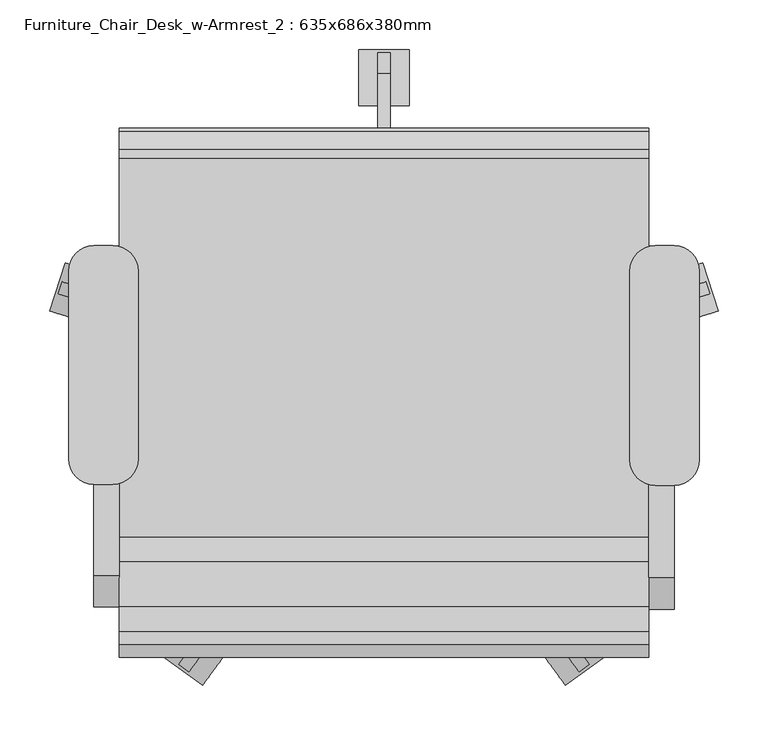
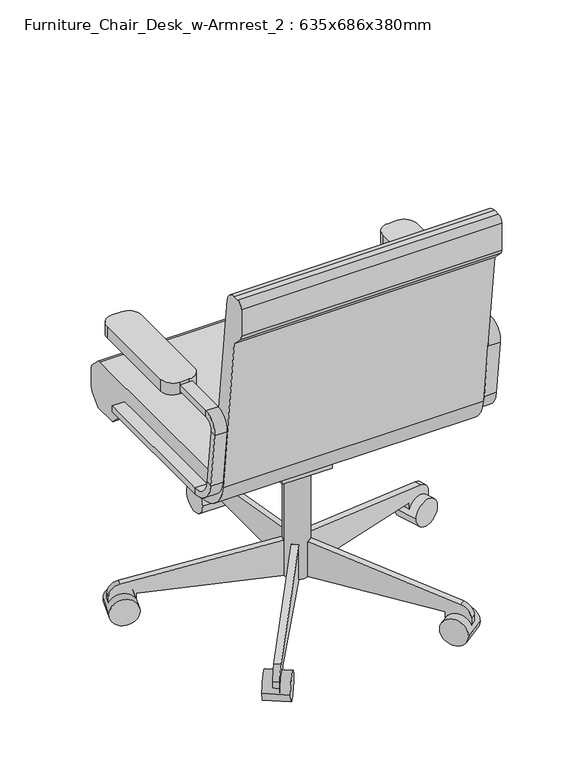
"""IFC4 building model written with IfcOpenShell, lengths in millimetres: furniture geometry, Furniture_Chair_Desk_w-Armrest_2 : 635x686x380mm."""

from ifc_helpers import new_model, si_unit, point, frame, frame_2d, origin, place, context, project, spatial, polyline, circle_curve, trimmed, segment, composite_curve, outline, extrude, source, transform, mapped, element, save
from ifc_brep_helpers import plane_surface, cylinder_surface, revolved_surface, advanced_brep


def furniture_chair_desk_w_armrest_2_635x686x380mm_bb362225(model_context):
    return source(origin(), model_context, "Body", "SolidModel", [
        extrude(outline(composite_curve([segment(polyline([(-126.2050455, 457.2), (255.0102301, 457.2)]), True, "CONTINUOUS"), segment(trimmed(circle_curve(frame_2d((255.0102301, 444.5)), 12.7), [point((255.0102301, 457.2))], [point((263.9604301, 453.510212))], False, "CARTESIAN"), True, "CONTINUOUS"), segment(polyline([(263.9604301, 453.510212), (281.8961016, 435.6939999)]), True, "CONTINUOUS"), segment(trimmed(circle_curve(frame_2d((272.9459016, 426.6837879)), 12.7), [point((281.8961016, 435.6939999))], [point((285.6459016, 426.6837879))], False, "CARTESIAN"), True, "CONTINUOUS"), segment(polyline([(285.6459016, 426.6837879), (285.6459016, 391.6405184)]), True, "CONTINUOUS"), segment(trimmed(circle_curve(frame_2d((260.2459016, 391.6405184)), 25.4), [point((285.6459016, 391.6405184))], [point((278.2663256, 373.7401184))], False, "CARTESIAN"), True, "CONTINUOUS"), segment(polyline([(278.2663256, 373.7401184), (260.2470284, 355.6), (209.4470284, 355.6), (181.0744602, 383.7835944), (-107.1089978, 383.7835944)]), True, "CONTINUOUS"), segment(trimmed(circle_curve(frame_2d((-107.1089978, 459.9835944)), 76.2), [point((-107.1089978, 383.7835944))], [point((-182.7870738, 451.0802913))], False, "CARTESIAN"), True, "CONTINUOUS"), segment(polyline([(-182.7870738, 451.0802913), (-222.3540984, 787.4), (-244.0343545, 809.0802561)]), True, "CONTINUOUS"), segment(trimmed(circle_curve(frame_2d((-235.0540984, 818.0605122)), 12.7), [point((-244.0343545, 809.0802561))], [point((-247.7540984, 818.0605122))], False, "CARTESIAN"), True, "CONTINUOUS"), segment(polyline([(-247.7540984, 818.0605122), (-247.7540984, 876.3)]), True, "CONTINUOUS"), segment(trimmed(circle_curve(frame_2d((-235.0540984, 876.3)), 12.7), [point((-247.7540984, 876.3))], [point((-235.0540984, 889.0))], False, "CARTESIAN"), True, "CONTINUOUS"), segment(polyline([(-235.0540984, 889.0), (-222.1789239, 889.0)]), True, "CONTINUOUS"), segment(trimmed(circle_curve(frame_2d((-222.1789239, 863.6)), 25.4), [point((-222.1789239, 889.0))], [point((-196.9528985, 866.5677677))], False, "CARTESIAN"), True, "CONTINUOUS"), segment(polyline([(-196.9528985, 866.5677677), (-151.4310708, 479.6322323)]), True, "CONTINUOUS"), segment(trimmed(circle_curve(frame_2d((-126.2050455, 482.6)), 25.4), [point((-151.4310708, 479.6322323))], [point((-126.2050455, 457.2))], True, "CARTESIAN"), True, "CONTINUOUS")], self_intersect=False)), frame((-125.7091803, 0.0, 0.0), z_axis=(1.0, 0.0, 0.0), x_axis=(0.0, 1.0, 0.0)), (0.0, 0.0, 1.0), 533.4),
        extrude(outline(polyline([(69.7459016, 383.7835944), (69.7459016, 371.0835944), (18.9459016, 283.0954134), (-19.1540984, 283.0954134), (-19.1540984, 383.7835944), (69.7459016, 383.7835944)])), frame((90.1908197, 0.0, 0.0), z_axis=(1.0, 0.0, 0.0), x_axis=(0.0, 1.0, 0.0)), (0.0, 0.0, 1.0), 101.6),
        extrude(outline(composite_curve([segment(polyline([(311.0459016, 53.5835944), (18.9459016, 53.5835944), (18.9459016, 129.7835944), (44.3459016, 129.7835944), (340.8565654, 77.5007643)]), True, "CONTINUOUS"), segment(trimmed(circle_curve(frame_2d((336.4459016, 52.4866474)), 25.4), [point((340.8565654, 77.5007643))], [point((361.8459016, 52.4866474))], False, "CARTESIAN"), True, "CONTINUOUS"), segment(polyline([(361.8459016, 52.4866474), (361.8459016, 28.1835944), (311.0459016, 28.1835944), (311.0459016, 53.5835944)]), True, "CONTINUOUS")], self_intersect=False)), frame((134.6408197, 0.0, 0.0), z_axis=(1.0, 0.0, 0.0), x_axis=(0.0, 1.0, 0.0)), (0.0, 0.0, 1.0), 12.7),
        extrude(outline(composite_curve([segment(trimmed(circle_curve(frame_2d((336.4459016, 28.1835944)), 28.2002727), [point((308.2456289, 28.1835944))], [point((364.6461744, 28.1835944))], False, "CARTESIAN"), True, "CONTINUOUS"), segment(trimmed(circle_curve(frame_2d((336.4459016, 28.1835944)), 28.2002727), [point((364.6461744, 28.1835944))], [point((308.2456289, 28.1835944))], False, "CARTESIAN"), True, "CONTINUOUS")], self_intersect=False)), frame((115.5908197, 0.0, 0.0), z_axis=(1.0, 0.0, 0.0), x_axis=(0.0, 1.0, 0.0)), (0.0, 0.0, 1.0), 50.8),
        extrude(outline(composite_curve([segment(polyline([(25.4, 0.0), (25.4, 292.1000001), (101.6, 292.1000001), (101.6, 266.7), (49.3171699, -29.8106636)]), True, "CONTINUOUS"), segment(trimmed(circle_curve(frame_2d((24.303053, -25.4)), 25.4), [point((49.3171699, -29.8106636))], [point((24.303053, -50.8))], False, "CARTESIAN"), True, "CONTINUOUS"), segment(polyline([(24.303053, -50.8), (0.0, -50.8), (0.0, 0.0), (25.4, 0.0)]), True, "CONTINUOUS")], self_intersect=False)), frame((-138.7750467, 103.1705568, 28.1835944), z_axis=(0.3090169943749487, 0.9510565162951532, 0.0), x_axis=(0.0, 0.0, 1.0)), (0.0, 0.0, 1.0), 12.7),
        extrude(outline(composite_curve([segment(trimmed(circle_curve(frame_2d((0.0, -28.2002727)), 28.2002727), [point((0.0, -56.4005454))], [point((0.0, 0.0))], False, "CARTESIAN"), True, "CONTINUOUS"), segment(trimmed(circle_curve(frame_2d((0.0, -28.2002727)), 28.2002727), [point((0.0, 0.0))], [point((0.0, -56.4005454))], False, "CARTESIAN"), True, "CONTINUOUS")], self_intersect=False)), frame((-195.638709, 101.6163254, 28.1835944), z_axis=(0.3090169943749487, 0.9510565162951532, 0.0), x_axis=(0.0, 0.0, -1.0)), (0.0, 0.0, 1.0), 50.8),
        extrude(outline(composite_curve([segment(polyline([(25.4, 0.0), (25.4, 292.1), (101.6, 292.1), (101.6, 266.7), (49.3171699, -29.8106637)]), True, "CONTINUOUS"), segment(trimmed(circle_curve(frame_2d((24.303053, -25.3999999)), 25.4), [point((49.3171699, -29.8106637))], [point((24.303053, -50.8))], False, "CARTESIAN"), True, "CONTINUOUS"), segment(polyline([(24.303053, -50.8), (0.0, -50.8), (0.0, 0.0), (25.4, 0.0)]), True, "CONTINUOUS")], self_intersect=False)), frame((-25.5639946, -221.1003988, 28.1835944), z_axis=(-0.8090169943749459, 0.5877852522924754, 0.0), x_axis=(0.0, 0.0, 1.0)), (0.0, 0.0, 1.0), 12.7),
        extrude(outline(composite_curve([segment(trimmed(circle_curve(frame_2d((0.0, -28.2002727)), 28.2002727), [point((0.0, -56.4005455))], [point((0.0, 0.0))], False, "CARTESIAN"), True, "CONTINUOUS"), segment(trimmed(circle_curve(frame_2d((0.0, -28.2002727)), 28.2002727), [point((0.0, 0.0))], [point((0.0, -56.4005455))], False, "CARTESIAN"), True, "CONTINUOUS")], self_intersect=False)), frame((-41.6576707, -275.6612394, 28.1835944), z_axis=(-0.8090169943749458, 0.5877852522924754, 0.0), x_axis=(0.0, 0.0, -1.0)), (0.0, 0.0, 1.0), 50.8),
        extrude(outline(composite_curve([segment(polyline([(-25.4, 0.0), (0.0, 0.0), (0.0, -50.8), (-24.303053, -50.8)]), True, "CONTINUOUS"), segment(trimmed(circle_curve(frame_2d((-24.303053, -25.3999999)), 25.4), [point((-24.303053, -50.8))], [point((-49.3171699, -29.8106636))], False, "CARTESIAN"), True, "CONTINUOUS"), segment(polyline([(-49.3171699, -29.8106636), (-101.6, 266.7), (-101.6, 292.1), (-25.4, 292.1), (-25.4, 0.0)]), True, "CONTINUOUS")], self_intersect=False)), frame((307.545634, -221.1003988, 28.1835944), z_axis=(0.8090169943749499, 0.5877852522924699, 0.0), x_axis=(0.0, 0.0, -1.0)), (0.0, 0.0, 1.0), 12.7),
        extrude(outline(composite_curve([segment(trimmed(circle_curve(frame_2d((0.0, -28.2002727)), 28.2002727), [point((0.0, -56.4005455))], [point((0.0, 0.0))], False, "CARTESIAN"), True, "CONTINUOUS"), segment(trimmed(circle_curve(frame_2d((0.0, -28.2002727)), 28.2002727), [point((0.0, 0.0))], [point((0.0, -56.4005455))], False, "CARTESIAN"), True, "CONTINUOUS")], self_intersect=False)), frame((323.63931, -275.6612394, 28.1835944), z_axis=(0.8090169943749499, 0.5877852522924699, 0.0), x_axis=(0.0, 0.0, 1.0)), (0.0, 0.0, 1.0), 50.8),
        extrude(outline(composite_curve([segment(polyline([(-25.4, 0.0), (0.0, 0.0), (0.0, -50.8), (-24.303053, -50.8)]), True, "CONTINUOUS"), segment(trimmed(circle_curve(frame_2d((-24.303053, -25.4)), 25.4), [point((-24.303053, -50.8))], [point((-49.3171699, -29.8106637))], False, "CARTESIAN"), True, "CONTINUOUS"), segment(polyline([(-49.3171699, -29.8106637), (-101.6, 266.7), (-101.6, 292.1), (-25.4, 292.1), (-25.4, 0.0)]), True, "CONTINUOUS")], self_intersect=False)), frame((420.756686, 103.1705568, 28.1835944), z_axis=(-0.3090169943749423, 0.9510565162951553, 0.0), x_axis=(0.0, 0.0, -1.0)), (0.0, 0.0, 1.0), 12.7),
        extrude(outline(composite_curve([segment(trimmed(circle_curve(frame_2d((0.0, -28.2002727)), 28.2002727), [point((0.0, -56.4005455))], [point((0.0, 0.0))], False, "CARTESIAN"), True, "CONTINUOUS"), segment(trimmed(circle_curve(frame_2d((0.0, -28.2002727)), 28.2002727), [point((0.0, 0.0))], [point((0.0, -56.4005455))], False, "CARTESIAN"), True, "CONTINUOUS")], self_intersect=False)), frame((477.6203484, 101.6163254, 28.1835944), z_axis=(-0.3090169943749423, 0.9510565162951553, 0.0), x_axis=(0.0, 0.0, 1.0)), (0.0, 0.0, 1.0), 50.8),
        extrude(outline(composite_curve([segment(trimmed(circle_curve(frame_2d((140.9908197, 18.9459016)), 25.4), [point((115.5908197, 18.9459016))], [point((166.3908197, 18.9459016))], False, "CARTESIAN"), True, "CONTINUOUS"), segment(trimmed(circle_curve(frame_2d((140.9908197, 18.9459016)), 25.4), [point((166.3908197, 18.9459016))], [point((115.5908197, 18.9459016))], False, "CARTESIAN"), True, "CONTINUOUS")], self_intersect=False)), frame((0.0, 0.0, 53.5835944), z_axis=(0.0, 0.0, 1.0), x_axis=(1.0, 0.0, 0.0)), (0.0, 0.0, 1.0), 330.5914056),
        advanced_brep(
        [(433.0908197, 167.0319091, 425.45), (433.0908197, 167.0319091, 412.75), (407.6908197, 167.0319091, 412.75), (407.6908197, 167.0319091, 425.45), (433.0908197, -128.329278, 425.45), (433.0908197, -128.329278, 412.75), (407.6908197, -128.329278, 412.75), (407.6908197, -128.329278, 425.45), (433.0908197, -185.0878351, 463.2225227), (433.0908197, -172.4748224, 464.7064065), (407.6908197, -185.0878351, 463.2225227), (407.6908197, -172.4748224, 464.7064065), (433.0908197, -186.2710303, 581.9741742), (433.0908197, -198.884043, 580.4902904), (407.6908197, -198.884043, 580.4902904), (407.6908197, -186.2710303, 581.9741742), (433.0908197, -167.3515113, 615.95), (433.0908197, -167.3515113, 603.25), (407.6908197, -167.3515113, 615.95), (407.6908197, -167.3515113, 603.25), (433.0908197, 18.9459016, 603.25), (407.6908197, 18.9459016, 603.25), (407.6908197, 18.9459016, 615.95), (433.0908197, 18.9459016, 615.95)],
        [
            (0, 1),
            (1, 2),
            (2, 3),
            (3, 0),
            (0, 4),
            (4, 5),
            (5, 1),
            (5, 6),
            (6, 2),
            (6, 7),
            (7, 3),
            (7, 4),
            (8, 5, circle_curve(frame((433.0908197, -128.329278, 469.9), z_axis=(1.0, 0.0, 0.0), x_axis=(0.0, 0.0, -1.0)), 57.15)),
            (4, 9, circle_curve(frame((433.0908197, -128.329278, 469.9), z_axis=(-1.0, 0.0, 0.0), x_axis=(0.0, 0.0, -1.0)), 44.45)),
            (9, 8),
            (10, 6, circle_curve(frame((407.6908197, -128.329278, 469.9), z_axis=(1.0, 0.0, 0.0), x_axis=(0.0, 0.0, -1.0)), 57.15)),
            (8, 10),
            (11, 7, circle_curve(frame((407.6908197, -128.329278, 469.9), z_axis=(1.0, 0.0, 0.0), x_axis=(0.0, 0.0, -1.0)), 44.45)),
            (10, 11),
            (11, 9),
            (9, 12),
            (12, 13),
            (13, 8),
            (13, 14),
            (14, 10),
            (14, 15),
            (15, 11),
            (15, 12),
            (16, 13, circle_curve(frame((433.0908197, -167.3515113, 584.2), z_axis=(1.0, 0.0, 0.0), x_axis=(0.0, -0.9931506043228767, -0.1168412475673929)), 31.75)),
            (12, 17, circle_curve(frame((433.0908197, -167.3515113, 584.2), z_axis=(-1.0, 0.0, 0.0), x_axis=(0.0, -0.9931506043228767, -0.1168412475673929)), 19.05)),
            (17, 16),
            (18, 14, circle_curve(frame((407.6908197, -167.3515113, 584.2), z_axis=(1.0, 0.0, 0.0), x_axis=(0.0, -0.9931506043228767, -0.1168412475673929)), 31.75)),
            (16, 18),
            (19, 15, circle_curve(frame((407.6908197, -167.3515113, 584.2), z_axis=(1.0, 0.0, 0.0), x_axis=(0.0, -0.9931506043228767, -0.1168412475673929)), 19.05)),
            (18, 19),
            (19, 17),
            (20, 21),
            (21, 22),
            (22, 23),
            (23, 20),
            (17, 20),
            (23, 16),
            (22, 18),
            (21, 19),
        ],
        [
            plane_surface(frame((406.191788, 167.0319091, 419.1), z_axis=(0.0, 1.0, 0.0), x_axis=(0.0, 0.0, -1.0))),
            plane_surface(frame((433.0908197, 167.0319091, 425.45), z_axis=(1.0, 0.0, 0.0), x_axis=(0.0, -1.0, 0.0))),
            plane_surface(frame((433.0908197, 167.0319091, 412.75), z_axis=(0.0, 0.0, -1.0), x_axis=(0.0, -1.0, 0.0))),
            plane_surface(frame((407.6908197, 167.0319091, 412.75), z_axis=(-1.0, 0.0, 0.0), x_axis=(0.0, -1.0, 0.0))),
            plane_surface(frame((407.6908197, 167.0319091, 425.45), z_axis=(0.0, 0.0, 1.0), x_axis=(0.0, -1.0, 0.0))),
            plane_surface(frame((433.0908197, -128.329278, 469.9), z_axis=(1.0, 0.0, 0.0), x_axis=(0.0, 0.0, -1.0))),
            cylinder_surface(frame((420.3908197, -128.329278, 469.9), z_axis=(-1.0, 0.0, 0.0), x_axis=(0.0, 0.0, -1.0)), 57.15),
            plane_surface(frame((407.6908197, -128.329278, 469.9), z_axis=(-1.0, 0.0, 0.0), x_axis=(0.0, 0.0, -1.0))),
            revolved_surface(polyline([(407.6908197, -128.329278, 425.45), (433.0908197, -128.329278, 425.45)]), (420.3908197, -128.329278, 469.9), (-1.0, 0.0, 0.0)),
            plane_surface(frame((433.0908197, -172.4748224, 464.7064065), z_axis=(1.0, 0.0, 0.0), x_axis=(0.0, -0.11684124756738626, 0.9931506043228775))),
            plane_surface(frame((433.0908197, -185.0878351, 463.2225227), z_axis=(0.0, -0.9931506043228775, -0.11684124756738655), x_axis=(0.0, -0.11684124756738655, 0.9931506043228775))),
            plane_surface(frame((407.6908197, -185.0878351, 463.2225227), z_axis=(-1.0, 0.0, 0.0), x_axis=(0.0, -0.11684124756738626, 0.9931506043228775))),
            plane_surface(frame((407.6908197, -172.4748224, 464.7064065), z_axis=(0.0, 0.9931506043228775, 0.11684124756738626), x_axis=(0.0, -0.11684124756738626, 0.9931506043228775))),
            plane_surface(frame((433.0908197, -167.3515113, 584.2), z_axis=(1.0, 0.0, 0.0), x_axis=(0.0, -0.9931506043228767, -0.1168412475673929))),
            cylinder_surface(frame((420.3908197, -167.3515113, 584.2), z_axis=(-1.0, 0.0, 0.0), x_axis=(0.0, -0.9931506043228767, -0.1168412475673929)), 31.75),
            plane_surface(frame((407.6908197, -167.3515113, 584.2), z_axis=(-1.0, 0.0, 0.0), x_axis=(0.0, -0.9931506043228767, -0.1168412475673929))),
            revolved_surface(polyline([(407.6908197, -186.2710303123508, 581.9741742338412), (433.0908197, -186.2710303123508, 581.9741742338412)]), (420.3908197, -167.3515113, 584.2), (-1.0, 0.0, 0.0)),
            plane_surface(frame((406.191788, 18.9459016, 609.6), z_axis=(0.0, 1.0, 0.0), x_axis=(0.0, 0.0, 1.0))),
            plane_surface(frame((433.0908197, -167.3515113, 603.25), z_axis=(1.0, 0.0, 0.0), x_axis=(0.0, 1.0, 0.0))),
            plane_surface(frame((433.0908197, -167.3515113, 615.95), z_axis=(0.0, 0.0, 1.0), x_axis=(0.0, 1.0, 0.0))),
            plane_surface(frame((407.6908197, -167.3515113, 615.95), z_axis=(-1.0, 0.0, 0.0), x_axis=(0.0, 1.0, 0.0))),
            plane_surface(frame((407.6908197, -167.3515113, 603.25), z_axis=(0.0, 0.0, -1.0), x_axis=(0.0, 1.0, 0.0))),
        ],
        [
            (0, [[1, 2, 3, 4]]),
            (1, [[-1, 5, 6, 7]]),
            (2, [[-2, -7, 8, 9]]),
            (3, [[-3, -9, 10, 11]]),
            (4, [[-4, -11, 12, -5]]),
            (5, [[13, -6, 14, 15]]),
            (6, [[16, -8, -13, 17]]),
            (7, [[18, -10, -16, 19]]),
            (8, [[-14, -12, -18, 20]]),
            (9, [[-15, 21, 22, 23]]),
            (10, [[-17, -23, 24, 25]]),
            (11, [[-19, -25, 26, 27]]),
            (12, [[-20, -27, 28, -21]]),
            (13, [[29, -22, 30, 31]]),
            (14, [[32, -24, -29, 33]]),
            (15, [[34, -26, -32, 35]]),
            (16, [[-30, -28, -34, 36]]),
            (17, [[37, 38, 39, 40]]),
            (18, [[-31, 41, -40, 42]]),
            (19, [[-33, -42, -39, 43]]),
            (20, [[-35, -43, -38, 44]]),
            (21, [[-36, -44, -37, -41]]),
        ],
    ),
        advanced_brep(
        [(-151.1091803, 167.0319091, 412.75), (-151.1091803, 167.0319091, 425.45), (-125.7091803, 167.0319091, 425.45), (-125.7091803, 167.0319091, 412.75), (-151.1091803, -126.2388651, 412.75), (-151.1091803, -126.2388651, 425.45), (-125.7091803, -126.2388651, 425.45), (-125.7091803, -126.2388651, 412.75), (-151.1091803, -170.3844094, 464.7064065), (-151.1091803, -182.9974221, 463.2225227), (-125.7091803, -170.3844094, 464.7064065), (-125.7091803, -182.9974221, 463.2225227), (-151.1091803, -196.7936301, 580.4902904), (-151.1091803, -184.1806174, 581.9741742), (-125.7091803, -184.1806174, 581.9741742), (-125.7091803, -196.7936301, 580.4902904), (-151.1091803, -165.2610984, 603.25), (-151.1091803, -165.2610984, 615.95), (-125.7091803, -165.2610984, 603.25), (-125.7091803, -165.2610984, 615.95), (-151.1091803, 18.9459016, 615.95), (-125.7091803, 18.9459016, 615.95), (-125.7091803, 18.9459016, 603.25), (-151.1091803, 18.9459016, 603.25)],
        [
            (0, 1),
            (1, 2),
            (2, 3),
            (3, 0),
            (0, 4),
            (4, 5),
            (5, 1),
            (5, 6),
            (6, 2),
            (6, 7),
            (7, 3),
            (7, 4),
            (8, 5, circle_curve(frame((-151.1091803, -126.2388651, 469.9), z_axis=(1.0, 0.0, 0.0), x_axis=(0.0, 0.0, -1.0)), 44.45)),
            (4, 9, circle_curve(frame((-151.1091803, -126.2388651, 469.9), z_axis=(-1.0, 0.0, 0.0), x_axis=(0.0, 0.0, -1.0)), 57.15)),
            (9, 8),
            (10, 6, circle_curve(frame((-125.7091803, -126.2388651, 469.9), z_axis=(1.0, 0.0, 0.0), x_axis=(0.0, 0.0, -1.0)), 44.45)),
            (8, 10),
            (11, 7, circle_curve(frame((-125.7091803, -126.2388651, 469.9), z_axis=(1.0, 0.0, 0.0), x_axis=(0.0, 0.0, -1.0)), 57.15)),
            (10, 11),
            (11, 9),
            (9, 12),
            (12, 13),
            (13, 8),
            (13, 14),
            (14, 10),
            (14, 15),
            (15, 11),
            (15, 12),
            (16, 13, circle_curve(frame((-151.1091803, -165.2610984, 584.2), z_axis=(1.0, 0.0, 0.0), x_axis=(0.0, -0.9931506043228768, -0.11684124756739202)), 19.05)),
            (12, 17, circle_curve(frame((-151.1091803, -165.2610984, 584.2), z_axis=(-1.0, 0.0, 0.0), x_axis=(0.0, -0.9931506043228768, -0.11684124756739202)), 31.75)),
            (17, 16),
            (18, 14, circle_curve(frame((-125.7091803, -165.2610984, 584.2), z_axis=(1.0, 0.0, 0.0), x_axis=(0.0, -0.9931506043228768, -0.11684124756739202)), 19.05)),
            (16, 18),
            (19, 15, circle_curve(frame((-125.7091803, -165.2610984, 584.2), z_axis=(1.0, 0.0, 0.0), x_axis=(0.0, -0.9931506043228768, -0.11684124756739202)), 31.75)),
            (18, 19),
            (19, 17),
            (20, 21),
            (21, 22),
            (22, 23),
            (23, 20),
            (17, 20),
            (23, 16),
            (22, 18),
            (21, 19),
        ],
        [
            plane_surface(frame((-152.608212, 167.0319091, 419.1), z_axis=(0.0, 1.0, 0.0), x_axis=(0.0, 0.0, -1.0))),
            plane_surface(frame((-151.1091803, 167.0319091, 412.75), z_axis=(-1.0, 0.0, 0.0), x_axis=(0.0, -1.0, 0.0))),
            plane_surface(frame((-151.1091803, 167.0319091, 425.45), z_axis=(0.0, 0.0, 1.0), x_axis=(0.0, -1.0, 0.0))),
            plane_surface(frame((-125.7091803, 167.0319091, 425.45), z_axis=(1.0, 0.0, 0.0), x_axis=(0.0, -1.0, 0.0))),
            plane_surface(frame((-125.7091803, 167.0319091, 412.75), z_axis=(0.0, 0.0, -1.0), x_axis=(0.0, -1.0, 0.0))),
            plane_surface(frame((-151.1091803, -126.2388651, 469.9), z_axis=(-1.0, 0.0, 0.0), x_axis=(0.0, 0.0, -1.0))),
            revolved_surface(polyline([(-151.1091803, -126.2388651, 425.45), (-125.7091803, -126.2388651, 425.45)]), (-138.4091803, -126.2388651, 469.9), (-1.0, 0.0, 0.0)),
            plane_surface(frame((-125.7091803, -126.2388651, 469.9), z_axis=(1.0, 0.0, 0.0), x_axis=(0.0, 0.0, -1.0))),
            cylinder_surface(frame((-138.4091803, -126.2388651, 469.9), z_axis=(-1.0, 0.0, 0.0), x_axis=(0.0, 0.0, -1.0)), 57.15),
            plane_surface(frame((-151.1091803, -182.9974221, 463.2225227), z_axis=(-1.0, 0.0, 0.0), x_axis=(0.0, -0.1168412475673856, 0.9931506043228776))),
            plane_surface(frame((-151.1091803, -170.3844094, 464.7064065), z_axis=(0.0, 0.9931506043228776, 0.1168412475673856), x_axis=(0.0, -0.1168412475673856, 0.9931506043228776))),
            plane_surface(frame((-125.7091803, -170.3844094, 464.7064065), z_axis=(1.0, 0.0, 0.0), x_axis=(0.0, -0.1168412475673856, 0.9931506043228776))),
            plane_surface(frame((-125.7091803, -182.9974221, 463.2225227), z_axis=(0.0, -0.9931506043228776, -0.1168412475673856), x_axis=(0.0, -0.1168412475673856, 0.9931506043228776))),
            plane_surface(frame((-151.1091803, -165.2610984, 584.2), z_axis=(-1.0, 0.0, 0.0), x_axis=(0.0, -0.9931506043228768, -0.11684124756739202))),
            revolved_surface(polyline([(-151.1091803, -184.1806174123508, 581.9741742338413), (-125.7091803, -184.1806174123508, 581.9741742338413)]), (-138.4091803, -165.2610984, 584.2), (-1.0, 0.0, 0.0)),
            plane_surface(frame((-125.7091803, -165.2610984, 584.2), z_axis=(1.0, 0.0, 0.0), x_axis=(0.0, -0.9931506043228768, -0.11684124756739202))),
            cylinder_surface(frame((-138.4091803, -165.2610984, 584.2), z_axis=(-1.0, 0.0, 0.0), x_axis=(0.0, -0.9931506043228768, -0.11684124756739202)), 31.75),
            plane_surface(frame((-152.608212, 18.9459016, 609.6), z_axis=(0.0, 1.0, 0.0), x_axis=(0.0, 0.0, 1.0))),
            plane_surface(frame((-151.1091803, -165.2610984, 615.95), z_axis=(-1.0, 0.0, 0.0), x_axis=(0.0, 1.0, 0.0))),
            plane_surface(frame((-151.1091803, -165.2610984, 603.25), z_axis=(0.0, 0.0, -1.0), x_axis=(0.0, 1.0, 0.0))),
            plane_surface(frame((-125.7091803, -165.2610984, 603.25), z_axis=(1.0, 0.0, 0.0), x_axis=(0.0, 1.0, 0.0))),
            plane_surface(frame((-125.7091803, -165.2610984, 615.95), z_axis=(0.0, 0.0, 1.0), x_axis=(0.0, 1.0, 0.0))),
        ],
        [
            (0, [[1, 2, 3, 4]]),
            (1, [[-1, 5, 6, 7]]),
            (2, [[-2, -7, 8, 9]]),
            (3, [[-3, -9, 10, 11]]),
            (4, [[-4, -11, 12, -5]]),
            (5, [[13, -6, 14, 15]]),
            (6, [[16, -8, -13, 17]]),
            (7, [[18, -10, -16, 19]]),
            (8, [[-14, -12, -18, 20]]),
            (9, [[-15, 21, 22, 23]]),
            (10, [[-17, -23, 24, 25]]),
            (11, [[-19, -25, 26, 27]]),
            (12, [[-20, -27, 28, -21]]),
            (13, [[29, -22, 30, 31]]),
            (14, [[32, -24, -29, 33]]),
            (15, [[34, -26, -32, 35]]),
            (16, [[-30, -28, -34, 36]]),
            (17, [[37, 38, 39, 40]]),
            (18, [[-31, 41, -40, 42]]),
            (19, [[-33, -42, -39, 43]]),
            (20, [[-35, -43, -38, 44]]),
            (21, [[-36, -44, -37, -41]]),
        ],
    ),
        extrude(outline(composite_curve([segment(polyline([(433.0908197, -74.2028048), (414.0408197, -74.2028048)]), True, "CONTINUOUS"), segment(trimmed(circle_curve(frame_2d((414.0408197, -48.8028048)), 25.4), [point((414.0408197, -74.2028048))], [point((388.6408197, -48.8028048))], False, "CARTESIAN"), True, "CONTINUOUS"), segment(polyline([(388.6408197, -48.8028048), (388.6408197, 141.6319091)]), True, "CONTINUOUS"), segment(trimmed(circle_curve(frame_2d((414.0408197, 141.6319091)), 25.4), [point((388.6408197, 141.6319091))], [point((414.0408197, 167.0319091))], False, "CARTESIAN"), True, "CONTINUOUS"), segment(polyline([(414.0408197, 167.0319091), (433.0908197, 167.0319091)]), True, "CONTINUOUS"), segment(trimmed(circle_curve(frame_2d((433.0908197, 141.6319091)), 25.4), [point((433.0908197, 167.0319091))], [point((458.4908197, 141.6319091))], False, "CARTESIAN"), True, "CONTINUOUS"), segment(polyline([(458.4908197, 141.6319091), (458.4908197, -48.8028048)]), True, "CONTINUOUS"), segment(trimmed(circle_curve(frame_2d((433.0908197, -48.8028048)), 25.4), [point((458.4908197, -48.8028048))], [point((433.0908197, -74.2028048))], False, "CARTESIAN"), True, "CONTINUOUS")], self_intersect=False)), frame((0.0, 0.0, 596.9), z_axis=(0.0, 0.0, 1.0), x_axis=(1.0, 0.0, 0.0)), (0.0, 0.0, 1.0), 25.4),
        extrude(outline(composite_curve([segment(polyline([(-132.0591803, -73.1575984), (-151.1091803, -73.1575984)]), True, "CONTINUOUS"), segment(trimmed(circle_curve(frame_2d((-151.1091803, -47.7575984)), 25.4), [point((-151.1091803, -73.1575984))], [point((-176.5091803, -47.7575984))], False, "CARTESIAN"), True, "CONTINUOUS"), segment(polyline([(-176.5091803, -47.7575984), (-176.5091803, 141.6319091)]), True, "CONTINUOUS"), segment(trimmed(circle_curve(frame_2d((-151.1091803, 141.6319091)), 25.4), [point((-176.5091803, 141.6319091))], [point((-151.1091803, 167.0319091))], False, "CARTESIAN"), True, "CONTINUOUS"), segment(polyline([(-151.1091803, 167.0319091), (-132.0591803, 167.0319091)]), True, "CONTINUOUS"), segment(trimmed(circle_curve(frame_2d((-132.0591803, 141.6319091)), 25.4), [point((-132.0591803, 167.0319091))], [point((-106.6591803, 141.6319091))], False, "CARTESIAN"), True, "CONTINUOUS"), segment(polyline([(-106.6591803, 141.6319091), (-106.6591803, -47.7575984)]), True, "CONTINUOUS"), segment(trimmed(circle_curve(frame_2d((-132.0591803, -47.7575984)), 25.4), [point((-106.6591803, -47.7575984))], [point((-132.0591803, -73.1575984))], False, "CARTESIAN"), True, "CONTINUOUS")], self_intersect=False)), frame((0.0, 0.0, 596.9), z_axis=(0.0, 0.0, 1.0), x_axis=(1.0, 0.0, 0.0)), (0.0, 0.0, 1.0), 25.4),
    ])


if __name__ == "__main__":
    model = new_model("IFC4")
    model_context = context("Model", 3, world=origin())
    ifc_project = project(units=[si_unit("LENGTHUNIT", "METRE", prefix="MILLI")], contexts=[model_context])
    site = spatial("IfcSite", under=ifc_project)
    building = spatial("IfcBuilding", under=site)
    placement = place(None, origin())
    furniture_chair_desk_w_armrest_2_635x686x380mm_shape = furniture_chair_desk_w_armrest_2_635x686x380mm_bb362225(model_context)
    element("IfcFurniture", 1, ObjectType="Furniture_Chair_Desk_w-Armrest_2 : 635x686x380mm", at=placement, inside=building, context=model_context, shape_type="MappedRepresentation", body=[
        mapped(furniture_chair_desk_w_armrest_2_635x686x380mm_shape, transform((0.0, 0.0, 0.0), x_axis=(1.0, 0.0, 0.0), y_axis=(0.0, 1.0, 0.0), z_axis=(0.0, 0.0, 1.0))),
    ])
    save(model, "model.ifc")

# Revit data of these elements
# Type "Furniture_Chair_Desk_w-Armrest_2 : 635x686x380mm"
#   Assembly Code = "E2020200"
#   Material Base = Plastic - Black
#   Material Caster = Plastic - Black
#   Material Seat/Back = Textile - Slate Blue
#   Default Elevation = 0
# Element 1 (IfcFurniture, "Furniture_Chair_Desk_w-Armrest_2 : 635x686x380mm")
#   Materials on its faces: "Plastic - Black", "Textile - Slate Blue"
# Materials
#   "Plastic - Black": colour RGB 0 0 0, transparency 0
#   "Textile - Slate Blue": class "Fabric", colour RGB 98 102 118, transparency 0
